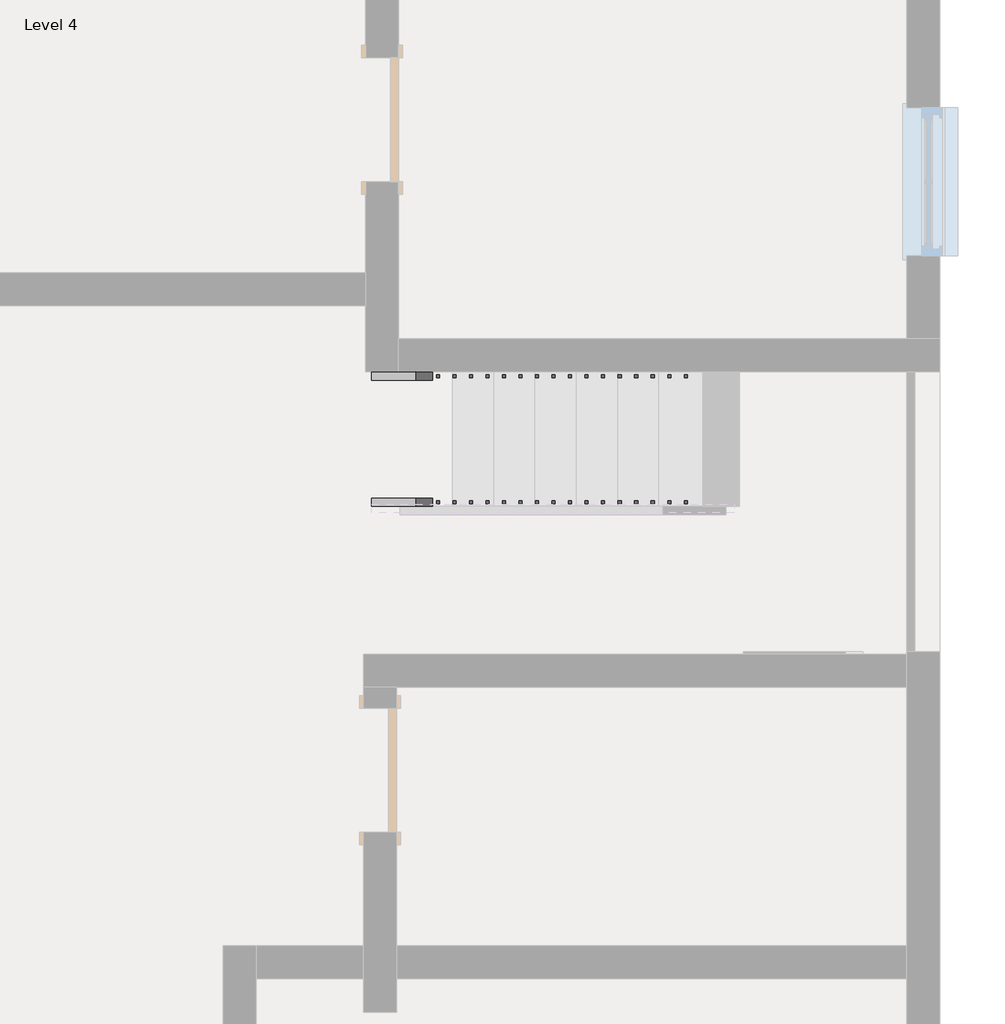
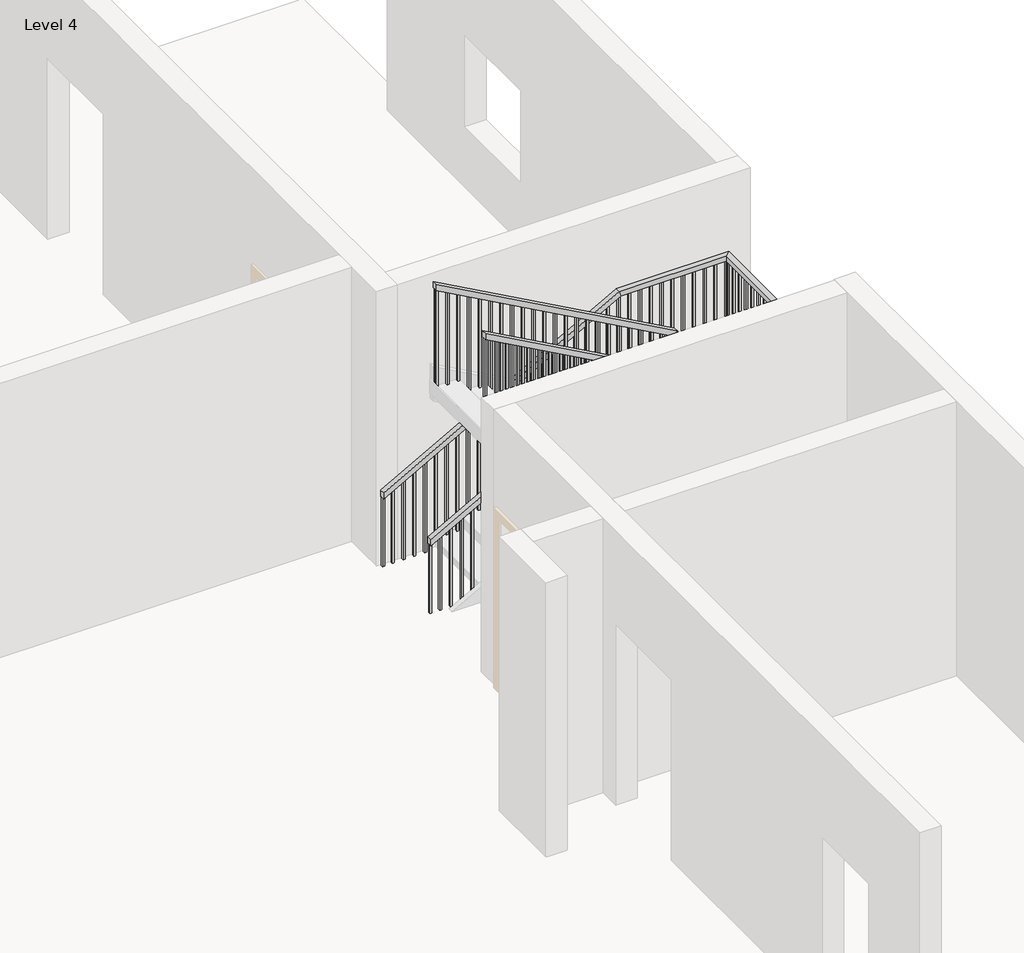
# One storey, part 3 of 4: 2 railings.
"""IFC4 building model written with IfcOpenShell, lengths in millimetres."""

from ifc_helpers import new_model, si_unit, frame, origin, place, context, project, spatial, polyline, outline, extrude, faceted_brep, element, save

model = new_model("IFC4")

# Units and contexts
model_context = context("Model", 3, world=origin())
ifc_project = project(units=[si_unit("LENGTHUNIT", "METRE", prefix="MILLI")], contexts=[model_context])

# Site, building, storey
site = spatial("IfcSite", under=ifc_project)
building = spatial("IfcBuilding", under=site)
storey = spatial("IfcBuildingStorey", under=building, Name="Level 4", Elevation=9144.0)

# Railings
placement = place(None, origin())
element("IfcRailing", 1, ObjectType="Handrail - Rectangular", at=placement, inside=storey, context=model_context, shape_type="SolidModel", body=[
    faceted_brep([(1537.1941283, 231.7547293, 10195.56), (1537.1941283, 231.7547293, 10137.4879132), (1537.1941283, 180.9547293, 10137.4879132), (1537.1941283, 180.9547293, 10195.56), (3765.8648053, 231.7547293, 11430.0), (3765.8648053, 180.9547293, 11430.0), (3765.8648053, 180.9547293, 11371.9279132), (3765.8648053, 231.7547293, 11371.9279132)], [[[0, 1, 2, 3]], [[4, 5, 6, 7]], [[1, 0, 4, 7]], [[2, 1, 7, 6]], [[3, 2, 6, 5]], [[0, 3, 5, 4]]]),
    faceted_brep([(3816.6648053, 231.7547293, 11430.0), (3816.6648053, 231.7547293, 11379.2), (3765.8648053, 231.7547293, 11379.2), (3765.8648053, 231.7547293, 11430.0), (3816.6648053, 142.8547293, 11430.0), (3765.8648053, 142.8547293, 11430.0), (3765.8648053, 92.0547293, 11379.2), (3816.6648053, 92.0547293, 11379.2)], [[[0, 1, 2, 3]], [[4, 5, 6, 7]], [[1, 0, 4, 7]], [[2, 1, 7, 6]], [[3, 2, 6, 5]], [[0, 3, 5, 4]]]),
    faceted_brep([(3816.6648053, 142.8547293, 11430.0), (3816.6648053, 92.0547293, 11379.2), (3765.8648053, 92.0547293, 11379.2), (3765.8648053, 142.8547293, 11430.0), (3816.6648053, 142.8547293, 11539.0223516), (3765.8648053, 142.8547293, 11509.0879132), (3765.8648053, 92.0547293, 11509.0879132), (3816.6648053, 92.0547293, 11539.0223516)], [[[0, 1, 2, 3]], [[4, 5, 6, 7]], [[1, 0, 4, 7]], [[2, 1, 7, 6]], [[3, 2, 6, 5]], [[0, 3, 5, 4]]]),
    faceted_brep([(3816.6648053, 92.0547293, 11539.0223516), (3765.8648053, 92.0547293, 11509.0879132), (3765.8648053, 142.8547293, 11509.0879132), (3816.6648053, 142.8547293, 11539.0223516), (1537.1941283, 92.0547293, 12801.6), (1537.1941283, 142.8547293, 12801.6), (1537.1941283, 142.8547293, 12743.5279132), (1537.1941283, 92.0547293, 12743.5279132)], [[[0, 1, 2, 3]], [[4, 5, 6, 7]], [[1, 0, 4, 7]], [[2, 1, 7, 6]], [[3, 2, 6, 5]], [[0, 3, 5, 4]]]),
    extrude(outline(polyline([(12727.7556667, 1565.5898053), (12738.3072849, 1546.5398053), (11750.04, 1546.5398053), (11750.04, 1565.5898053), (12727.7556667, 1565.5898053)])), frame((0.0, 107.9297293, 0.0), z_axis=(0.0, 1.0, 0.0), x_axis=(0.0, 0.0, 1.0)), (0.0, 0.0, 1.0), 19.05),
    extrude(outline(polyline([(12671.4803699, 1667.1898053), (12682.031988, 1648.1398053), (11750.04, 1648.1398053), (11750.04, 1667.1898053), (12671.4803699, 1667.1898053)])), frame((0.0, 107.9297293, 0.0), z_axis=(0.0, 1.0, 0.0), x_axis=(0.0, 0.0, 1.0)), (0.0, 0.0, 1.0), 19.05),
    extrude(outline(polyline([(12615.1609284, 1768.7898053), (12625.7125465, 1749.7398053), (11750.04, 1749.7398053), (11750.04, 1768.7898053), (12615.1609284, 1768.7898053)])), frame((0.0, 107.9297293, 0.0), z_axis=(0.0, 1.0, 0.0), x_axis=(0.0, 0.0, 1.0)), (0.0, 0.0, 1.0), 19.05),
    extrude(outline(polyline([(12558.9297761, 1870.3898053), (12569.4813943, 1851.3398053), (11612.88, 1851.3398053), (11612.88, 1870.3898053), (12558.9297761, 1870.3898053)])), frame((0.0, 107.9297293, 0.0), z_axis=(0.0, 1.0, 0.0), x_axis=(0.0, 0.0, 1.0)), (0.0, 0.0, 1.0), 19.05),
    extrude(outline(polyline([(12502.6544792, 1971.9898053), (12513.2060974, 1952.9398053), (11612.88, 1952.9398053), (11612.88, 1971.9898053), (12502.6544792, 1971.9898053)])), frame((0.0, 107.9297293, 0.0), z_axis=(0.0, 1.0, 0.0), x_axis=(0.0, 0.0, 1.0)), (0.0, 0.0, 1.0), 19.05),
    extrude(outline(polyline([(12446.3791823, 2073.5898053), (12456.9308005, 2054.5398053), (11475.72, 2054.5398053), (11475.72, 2073.5898053), (12446.3791823, 2073.5898053)])), frame((0.0, 107.9297293, 0.0), z_axis=(0.0, 1.0, 0.0), x_axis=(0.0, 0.0, 1.0)), (0.0, 0.0, 1.0), 19.05),
    extrude(outline(polyline([(12390.1038855, 2175.1898053), (12400.6555036, 2156.1398053), (11475.72, 2156.1398053), (11475.72, 2175.1898053), (12390.1038855, 2175.1898053)])), frame((0.0, 107.9297293, 0.0), z_axis=(0.0, 1.0, 0.0), x_axis=(0.0, 0.0, 1.0)), (0.0, 0.0, 1.0), 19.05),
    extrude(outline(polyline([(12333.8285886, 2276.7898053), (12344.3802067, 2257.7398053), (11475.72, 2257.7398053), (11475.72, 2276.7898053), (12333.8285886, 2276.7898053)])), frame((0.0, 107.9297293, 0.0), z_axis=(0.0, 1.0, 0.0), x_axis=(0.0, 0.0, 1.0)), (0.0, 0.0, 1.0), 19.05),
    extrude(outline(polyline([(12277.5532917, 2378.3898053), (12288.1049099, 2359.3398053), (11338.56, 2359.3398053), (11338.56, 2378.3898053), (12277.5532917, 2378.3898053)])), frame((0.0, 107.9297293, 0.0), z_axis=(0.0, 1.0, 0.0), x_axis=(0.0, 0.0, 1.0)), (0.0, 0.0, 1.0), 19.05),
    extrude(outline(polyline([(12221.2779948, 2479.9898053), (12231.829613, 2460.9398053), (11338.56, 2460.9398053), (11338.56, 2479.9898053), (12221.2779948, 2479.9898053)])), frame((0.0, 107.9297293, 0.0), z_axis=(0.0, 1.0, 0.0), x_axis=(0.0, 0.0, 1.0)), (0.0, 0.0, 1.0), 19.05),
    extrude(outline(polyline([(12165.0026979, 2581.5898053), (12175.5543161, 2562.5398053), (11201.4, 2562.5398053), (11201.4, 2581.5898053), (12165.0026979, 2581.5898053)])), frame((0.0, 107.9297293, 0.0), z_axis=(0.0, 1.0, 0.0), x_axis=(0.0, 0.0, 1.0)), (0.0, 0.0, 1.0), 19.05),
    extrude(outline(polyline([(12108.727401, 2683.1898053), (12119.2790192, 2664.1398053), (11201.4, 2664.1398053), (11201.4, 2683.1898053), (12108.727401, 2683.1898053)])), frame((0.0, 107.9297293, 0.0), z_axis=(0.0, 1.0, 0.0), x_axis=(0.0, 0.0, 1.0)), (0.0, 0.0, 1.0), 19.05),
    extrude(outline(polyline([(12052.4962488, 2784.7898053), (12063.0478669, 2765.7398053), (11201.4, 2765.7398053), (11201.4, 2784.7898053), (12052.4962488, 2784.7898053)])), frame((0.0, 107.9297293, 0.0), z_axis=(0.0, 1.0, 0.0), x_axis=(0.0, 0.0, 1.0)), (0.0, 0.0, 1.0), 19.05),
    extrude(outline(polyline([(11996.2209519, 2886.3898053), (12006.77257, 2867.3398053), (11064.24, 2867.3398053), (11064.24, 2886.3898053), (11996.2209519, 2886.3898053)])), frame((0.0, 107.9297293, 0.0), z_axis=(0.0, 1.0, 0.0), x_axis=(0.0, 0.0, 1.0)), (0.0, 0.0, 1.0), 19.05),
    extrude(outline(polyline([(11939.945655, 2987.9898053), (11950.4972732, 2968.9398053), (11064.24, 2968.9398053), (11064.24, 2987.9898053), (11939.945655, 2987.9898053)])), frame((0.0, 107.9297293, 0.0), z_axis=(0.0, 1.0, 0.0), x_axis=(0.0, 0.0, 1.0)), (0.0, 0.0, 1.0), 19.05),
    extrude(outline(polyline([(11883.6703581, 3089.5898053), (11894.2219763, 3070.5398053), (10927.08, 3070.5398053), (10927.08, 3089.5898053), (11883.6703581, 3089.5898053)])), frame((0.0, 107.9297293, 0.0), z_axis=(0.0, 1.0, 0.0), x_axis=(0.0, 0.0, 1.0)), (0.0, 0.0, 1.0), 19.05),
    extrude(outline(polyline([(11827.3950612, 3191.1898053), (11837.9466794, 3172.1398053), (10927.08, 3172.1398053), (10927.08, 3191.1898053), (11827.3950612, 3191.1898053)])), frame((0.0, 107.9297293, 0.0), z_axis=(0.0, 1.0, 0.0), x_axis=(0.0, 0.0, 1.0)), (0.0, 0.0, 1.0), 19.05),
    extrude(outline(polyline([(11771.1197643, 3292.7898053), (11781.6713825, 3273.7398053), (10927.08, 3273.7398053), (10927.08, 3292.7898053), (11771.1197643, 3292.7898053)])), frame((0.0, 107.9297293, 0.0), z_axis=(0.0, 1.0, 0.0), x_axis=(0.0, 0.0, 1.0)), (0.0, 0.0, 1.0), 19.05),
    extrude(outline(polyline([(11714.8444675, 3394.3898053), (11725.3960856, 3375.3398053), (10789.92, 3375.3398053), (10789.92, 3394.3898053), (11714.8444675, 3394.3898053)])), frame((0.0, 107.9297293, 0.0), z_axis=(0.0, 1.0, 0.0), x_axis=(0.0, 0.0, 1.0)), (0.0, 0.0, 1.0), 19.05),
    extrude(outline(polyline([(11658.5691706, 3495.9898053), (11669.1207888, 3476.9398053), (10789.92, 3476.9398053), (10789.92, 3495.9898053), (11658.5691706, 3495.9898053)])), frame((0.0, 107.9297293, 0.0), z_axis=(0.0, 1.0, 0.0), x_axis=(0.0, 0.0, 1.0)), (0.0, 0.0, 1.0), 19.05),
    extrude(outline(polyline([(11602.2938737, 3597.5898053), (11612.8454919, 3578.5398053), (10652.76, 3578.5398053), (10652.76, 3597.5898053), (11602.2938737, 3597.5898053)])), frame((0.0, 107.9297293, 0.0), z_axis=(0.0, 1.0, 0.0), x_axis=(0.0, 0.0, 1.0)), (0.0, 0.0, 1.0), 19.05),
    extrude(outline(polyline([(11546.0185768, 3699.1898053), (11556.570195, 3680.1398053), (10652.76, 3680.1398053), (10652.76, 3699.1898053), (11546.0185768, 3699.1898053)])), frame((0.0, 107.9297293, 0.0), z_axis=(0.0, 1.0, 0.0), x_axis=(0.0, 0.0, 1.0)), (0.0, 0.0, 1.0), 19.05),
    extrude(outline(polyline([(11380.8202537, 3781.9191283), (11370.2686355, 3762.8691283), (10515.6, 3762.8691283), (10515.6, 3781.9191283), (11380.8202537, 3781.9191283)])), frame((0.0, 196.8297293, 0.0), z_axis=(0.0, 1.0, 0.0), x_axis=(0.0, 0.0, 1.0)), (0.0, 0.0, 1.0), 19.05),
    extrude(outline(polyline([(11324.5449568, 3680.3191283), (11313.9933387, 3661.2691283), (10378.44, 3661.2691283), (10378.44, 3680.3191283), (11324.5449568, 3680.3191283)])), frame((0.0, 196.8297293, 0.0), z_axis=(0.0, 1.0, 0.0), x_axis=(0.0, 0.0, 1.0)), (0.0, 0.0, 1.0), 19.05),
    extrude(outline(polyline([(11268.2696599, 3578.7191283), (11257.7180418, 3559.6691283), (10378.44, 3559.6691283), (10378.44, 3578.7191283), (11268.2696599, 3578.7191283)])), frame((0.0, 196.8297293, 0.0), z_axis=(0.0, 1.0, 0.0), x_axis=(0.0, 0.0, 1.0)), (0.0, 0.0, 1.0), 19.05),
    extrude(outline(polyline([(11211.9943631, 3477.1191283), (11201.4427449, 3458.0691283), (10241.28, 3458.0691283), (10241.28, 3477.1191283), (11211.9943631, 3477.1191283)])), frame((0.0, 196.8297293, 0.0), z_axis=(0.0, 1.0, 0.0), x_axis=(0.0, 0.0, 1.0)), (0.0, 0.0, 1.0), 19.05),
    extrude(outline(polyline([(11155.7190662, 3375.5191283), (11145.167448, 3356.4691283), (10241.28, 3356.4691283), (10241.28, 3375.5191283), (11155.7190662, 3375.5191283)])), frame((0.0, 196.8297293, 0.0), z_axis=(0.0, 1.0, 0.0), x_axis=(0.0, 0.0, 1.0)), (0.0, 0.0, 1.0), 19.05),
    extrude(outline(polyline([(11099.4437693, 3273.9191283), (11088.8921511, 3254.8691283), (10104.12, 3254.8691283), (10104.12, 3273.9191283), (11099.4437693, 3273.9191283)])), frame((0.0, 196.8297293, 0.0), z_axis=(0.0, 1.0, 0.0), x_axis=(0.0, 0.0, 1.0)), (0.0, 0.0, 1.0), 19.05),
    extrude(outline(polyline([(11043.1684724, 3172.3191283), (11032.6168543, 3153.2691283), (10104.12, 3153.2691283), (10104.12, 3172.3191283), (11043.1684724, 3172.3191283)])), frame((0.0, 196.8297293, 0.0), z_axis=(0.0, 1.0, 0.0), x_axis=(0.0, 0.0, 1.0)), (0.0, 0.0, 1.0), 19.05),
    extrude(outline(polyline([(10986.8931755, 3070.7191283), (10976.3415574, 3051.6691283), (10104.12, 3051.6691283), (10104.12, 3070.7191283), (10986.8931755, 3070.7191283)])), frame((0.0, 196.8297293, 0.0), z_axis=(0.0, 1.0, 0.0), x_axis=(0.0, 0.0, 1.0)), (0.0, 0.0, 1.0), 19.05),
    extrude(outline(polyline([(10930.6178787, 2969.1191283), (10920.0662605, 2950.0691283), (9966.96, 2950.0691283), (9966.96, 2969.1191283), (10930.6178787, 2969.1191283)])), frame((0.0, 196.8297293, 0.0), z_axis=(0.0, 1.0, 0.0), x_axis=(0.0, 0.0, 1.0)), (0.0, 0.0, 1.0), 19.05),
    extrude(outline(polyline([(10874.3425818, 2867.5191283), (10863.7909636, 2848.4691283), (9966.96, 2848.4691283), (9966.96, 2867.5191283), (10874.3425818, 2867.5191283)])), frame((0.0, 196.8297293, 0.0), z_axis=(0.0, 1.0, 0.0), x_axis=(0.0, 0.0, 1.0)), (0.0, 0.0, 1.0), 19.05),
    extrude(outline(polyline([(10818.0672849, 2765.9191283), (10807.5156667, 2746.8691283), (9829.8, 2746.8691283), (9829.8, 2765.9191283), (10818.0672849, 2765.9191283)])), frame((0.0, 196.8297293, 0.0), z_axis=(0.0, 1.0, 0.0), x_axis=(0.0, 0.0, 1.0)), (0.0, 0.0, 1.0), 19.05),
    extrude(outline(polyline([(10761.791988, 2664.3191283), (10751.2403699, 2645.2691283), (9829.8, 2645.2691283), (9829.8, 2664.3191283), (10761.791988, 2664.3191283)])), frame((0.0, 196.8297293, 0.0), z_axis=(0.0, 1.0, 0.0), x_axis=(0.0, 0.0, 1.0)), (0.0, 0.0, 1.0), 19.05),
    extrude(outline(polyline([(10705.4725466, 2562.7191283), (10694.9209284, 2543.6691283), (9829.8, 2543.6691283), (9829.8, 2562.7191283), (10705.4725466, 2562.7191283)])), frame((0.0, 196.8297293, 0.0), z_axis=(0.0, 1.0, 0.0), x_axis=(0.0, 0.0, 1.0)), (0.0, 0.0, 1.0), 19.05),
    extrude(outline(polyline([(10649.2413943, 2461.1191283), (10638.6897761, 2442.0691283), (9692.64, 2442.0691283), (9692.64, 2461.1191283), (10649.2413943, 2461.1191283)])), frame((0.0, 196.8297293, 0.0), z_axis=(0.0, 1.0, 0.0), x_axis=(0.0, 0.0, 1.0)), (0.0, 0.0, 1.0), 19.05),
    extrude(outline(polyline([(10592.9660974, 2359.5191283), (10582.4144792, 2340.4691283), (9692.64, 2340.4691283), (9692.64, 2359.5191283), (10592.9660974, 2359.5191283)])), frame((0.0, 196.8297293, 0.0), z_axis=(0.0, 1.0, 0.0), x_axis=(0.0, 0.0, 1.0)), (0.0, 0.0, 1.0), 19.05),
    extrude(outline(polyline([(10536.6908005, 2257.9191283), (10526.1391823, 2238.8691283), (9555.48, 2238.8691283), (9555.48, 2257.9191283), (10536.6908005, 2257.9191283)])), frame((0.0, 196.8297293, 0.0), z_axis=(0.0, 1.0, 0.0), x_axis=(0.0, 0.0, 1.0)), (0.0, 0.0, 1.0), 19.05),
    extrude(outline(polyline([(10480.4155036, 2156.3191283), (10469.8638855, 2137.2691283), (9555.48, 2137.2691283), (9555.48, 2156.3191283), (10480.4155036, 2156.3191283)])), frame((0.0, 196.8297293, 0.0), z_axis=(0.0, 1.0, 0.0), x_axis=(0.0, 0.0, 1.0)), (0.0, 0.0, 1.0), 19.05),
    extrude(outline(polyline([(10424.1402067, 2054.7191283), (10413.5885886, 2035.6691283), (9555.48, 2035.6691283), (9555.48, 2054.7191283), (10424.1402067, 2054.7191283)])), frame((0.0, 196.8297293, 0.0), z_axis=(0.0, 1.0, 0.0), x_axis=(0.0, 0.0, 1.0)), (0.0, 0.0, 1.0), 19.05),
    extrude(outline(polyline([(10367.8649099, 1953.1191283), (10357.3132917, 1934.0691283), (9418.32, 1934.0691283), (9418.32, 1953.1191283), (10367.8649099, 1953.1191283)])), frame((0.0, 196.8297293, 0.0), z_axis=(0.0, 1.0, 0.0), x_axis=(0.0, 0.0, 1.0)), (0.0, 0.0, 1.0), 19.05),
    extrude(outline(polyline([(10311.589613, 1851.5191283), (10301.0379948, 1832.4691283), (9418.32, 1832.4691283), (9418.32, 1851.5191283), (10311.589613, 1851.5191283)])), frame((0.0, 196.8297293, 0.0), z_axis=(0.0, 1.0, 0.0), x_axis=(0.0, 0.0, 1.0)), (0.0, 0.0, 1.0), 19.05),
    extrude(outline(polyline([(10255.3143161, 1749.9191283), (10244.7626979, 1730.8691283), (9281.16, 1730.8691283), (9281.16, 1749.9191283), (10255.3143161, 1749.9191283)])), frame((0.0, 196.8297293, 0.0), z_axis=(0.0, 1.0, 0.0), x_axis=(0.0, 0.0, 1.0)), (0.0, 0.0, 1.0), 19.05),
    extrude(outline(polyline([(10199.0390192, 1648.3191283), (10188.487401, 1629.2691283), (9281.16, 1629.2691283), (9281.16, 1648.3191283), (10199.0390192, 1648.3191283)])), frame((0.0, 196.8297293, 0.0), z_axis=(0.0, 1.0, 0.0), x_axis=(0.0, 0.0, 1.0)), (0.0, 0.0, 1.0), 19.05),
    extrude(outline(polyline([(3781.7398053, 126.9797293), (3800.7898053, 126.9797293), (3800.7898053, 107.9297293), (3781.7398053, 107.9297293), (3781.7398053, 126.9797293)])), frame((0.0, 0.0, 10515.6), z_axis=(0.0, 0.0, 1.0), x_axis=(1.0, 0.0, 0.0)), (0.0, 0.0, 1.0), 863.6),
    extrude(outline(polyline([(11391.2725465, 3800.7898053), (11380.7209284, 3781.7398053), (10515.6, 3781.7398053), (10515.6, 3800.7898053), (11391.2725465, 3800.7898053)])), frame((0.0, 196.8297293, 0.0), z_axis=(0.0, 1.0, 0.0), x_axis=(0.0, 0.0, 1.0)), (0.0, 0.0, 1.0), 19.05),
    extrude(outline(polyline([(12732.9762951, 1556.2441283), (12743.5279132, 1537.1941283), (11750.04, 1537.1941283), (11750.04, 1556.2441283), (12732.9762951, 1556.2441283)])), frame((0.0, 107.9297293, 0.0), z_axis=(0.0, 1.0, 0.0), x_axis=(0.0, 0.0, 1.0)), (0.0, 0.0, 1.0), 19.05),
    extrude(outline(polyline([(10148.0395314, 1556.2441283), (10137.4879132, 1537.1941283), (9281.16, 1537.1941283), (9281.16, 1556.2441283), (10148.0395314, 1556.2441283)])), frame((0.0, 196.8297293, 0.0), z_axis=(0.0, 1.0, 0.0), x_axis=(0.0, 0.0, 1.0)), (0.0, 0.0, 1.0), 19.05),
])
element("IfcRailing", 2, ObjectType="Handrail - Rectangular", at=placement, inside=storey, context=model_context, shape_type="SolidModel", body=[
    faceted_brep([(1537.1941283, 1006.4547293, 10195.56), (1537.1941283, 1006.4547293, 10137.4879132), (1537.1941283, 955.6547293, 10137.4879132), (1537.1941283, 955.6547293, 10195.56), (3765.8648053, 1006.4547293, 11430.0), (3778.9939056, 1006.4547293, 11379.2), (3778.9939056, 955.6547293, 11379.2), (3765.8648053, 955.6547293, 11430.0), (4826.4941283, 1006.4547293, 11430.0), (4826.4941283, 1006.4547293, 11379.2), (4775.6941283, 955.6547293, 11379.2), (4775.6941283, 955.6547293, 11430.0), (4826.4941283, -714.2964201, 11430.0), (4826.4941283, -714.2964201, 11379.2), (4775.6941283, -663.4964201, 11379.2), (4775.6941283, -663.4964201, 11430.0), (4013.4948805, -714.2964201, 11430.0), (4000.3657803, -714.2964201, 11379.2), (4000.3657803, -663.4964201, 11379.2), (4013.4948805, -663.4964201, 11430.0), (1537.1941283, -714.2964201, 12801.6), (1537.1941283, -663.4964201, 12801.6), (1537.1941283, -663.4964201, 12743.5279132), (1537.1941283, -714.2964201, 12743.5279132)], [[[0, 1, 2, 3]], [[1, 0, 4, 5]], [[2, 1, 5, 6]], [[3, 2, 6, 7]], [[0, 3, 7, 4]], [[5, 4, 8, 9]], [[6, 5, 9, 10]], [[7, 6, 10, 11]], [[4, 7, 11, 8]], [[9, 8, 12, 13]], [[10, 9, 13, 14]], [[11, 10, 14, 15]], [[8, 11, 15, 12]], [[13, 12, 16, 17]], [[14, 13, 17, 18]], [[15, 14, 18, 19]], [[12, 15, 19, 16]], [[20, 21, 22, 23]], [[17, 16, 20, 23]], [[18, 17, 23, 22]], [[19, 18, 22, 21]], [[16, 19, 21, 20]]]),
    extrude(outline(polyline([(12741.7693102, 1540.3691283), (11750.04, 1540.3691283), (11750.04, 1559.4191283), (12731.2176921, 1559.4191283), (12741.7693102, 1540.3691283)])), frame((0.0, -698.4214201, 0.0), z_axis=(0.0, 1.0, 0.0), x_axis=(0.0, 0.0, 1.0)), (0.0, 0.0, 1.0), 19.05),
    extrude(outline(polyline([(12685.4940133, 1641.9691283), (11750.04, 1641.9691283), (11750.04, 1661.0191283), (12674.9423952, 1661.0191283), (12685.4940133, 1641.9691283)])), frame((0.0, -698.4214201, 0.0), z_axis=(0.0, 1.0, 0.0), x_axis=(0.0, 0.0, 1.0)), (0.0, 0.0, 1.0), 19.05),
    extrude(outline(polyline([(12629.2187165, 1743.5691283), (11750.04, 1743.5691283), (11750.04, 1762.6191283), (12618.6670983, 1762.6191283), (12629.2187165, 1743.5691283)])), frame((0.0, -698.4214201, 0.0), z_axis=(0.0, 1.0, 0.0), x_axis=(0.0, 0.0, 1.0)), (0.0, 0.0, 1.0), 19.05),
    extrude(outline(polyline([(12572.9434196, 1845.1691283), (11612.88, 1845.1691283), (11612.88, 1864.2191283), (12562.3918014, 1864.2191283), (12572.9434196, 1845.1691283)])), frame((0.0, -698.4214201, 0.0), z_axis=(0.0, 1.0, 0.0), x_axis=(0.0, 0.0, 1.0)), (0.0, 0.0, 1.0), 19.05),
    extrude(outline(polyline([(12516.6681227, 1946.7691283), (11612.88, 1946.7691283), (11612.88, 1965.8191283), (12506.1165045, 1965.8191283), (12516.6681227, 1946.7691283)])), frame((0.0, -698.4214201, 0.0), z_axis=(0.0, 1.0, 0.0), x_axis=(0.0, 0.0, 1.0)), (0.0, 0.0, 1.0), 19.05),
    extrude(outline(polyline([(12460.3928258, 2048.3691283), (11475.72, 2048.3691283), (11475.72, 2067.4191283), (12449.8412076, 2067.4191283), (12460.3928258, 2048.3691283)])), frame((0.0, -698.4214201, 0.0), z_axis=(0.0, 1.0, 0.0), x_axis=(0.0, 0.0, 1.0)), (0.0, 0.0, 1.0), 19.05),
    extrude(outline(polyline([(12404.1175289, 2149.9691283), (11475.72, 2149.9691283), (11475.72, 2169.0191283), (12393.5659108, 2169.0191283), (12404.1175289, 2149.9691283)])), frame((0.0, -698.4214201, 0.0), z_axis=(0.0, 1.0, 0.0), x_axis=(0.0, 0.0, 1.0)), (0.0, 0.0, 1.0), 19.05),
    extrude(outline(polyline([(12347.8422321, 2251.5691283), (11475.72, 2251.5691283), (11475.72, 2270.6191283), (12337.2906139, 2270.6191283), (12347.8422321, 2251.5691283)])), frame((0.0, -698.4214201, 0.0), z_axis=(0.0, 1.0, 0.0), x_axis=(0.0, 0.0, 1.0)), (0.0, 0.0, 1.0), 19.05),
    extrude(outline(polyline([(12291.5669352, 2353.1691283), (11338.56, 2353.1691283), (11338.56, 2372.2191283), (12281.015317, 2372.2191283), (12291.5669352, 2353.1691283)])), frame((0.0, -698.4214201, 0.0), z_axis=(0.0, 1.0, 0.0), x_axis=(0.0, 0.0, 1.0)), (0.0, 0.0, 1.0), 19.05),
    extrude(outline(polyline([(12235.2916383, 2454.7691283), (11338.56, 2454.7691283), (11338.56, 2473.8191283), (12224.7400201, 2473.8191283), (12235.2916383, 2454.7691283)])), frame((0.0, -698.4214201, 0.0), z_axis=(0.0, 1.0, 0.0), x_axis=(0.0, 0.0, 1.0)), (0.0, 0.0, 1.0), 19.05),
    extrude(outline(polyline([(12179.0163414, 2556.3691283), (11201.4, 2556.3691283), (11201.4, 2575.4191283), (12168.4647232, 2575.4191283), (12179.0163414, 2556.3691283)])), frame((0.0, -698.4214201, 0.0), z_axis=(0.0, 1.0, 0.0), x_axis=(0.0, 0.0, 1.0)), (0.0, 0.0, 1.0), 19.05),
    extrude(outline(polyline([(12122.7410445, 2657.9691283), (11201.4, 2657.9691283), (11201.4, 2677.0191283), (12112.1894264, 2677.0191283), (12122.7410445, 2657.9691283)])), frame((0.0, -698.4214201, 0.0), z_axis=(0.0, 1.0, 0.0), x_axis=(0.0, 0.0, 1.0)), (0.0, 0.0, 1.0), 19.05),
    extrude(outline(polyline([(12066.4657476, 2759.5691283), (11201.4, 2759.5691283), (11201.4, 2778.6191283), (12055.9141295, 2778.6191283), (12066.4657476, 2759.5691283)])), frame((0.0, -698.4214201, 0.0), z_axis=(0.0, 1.0, 0.0), x_axis=(0.0, 0.0, 1.0)), (0.0, 0.0, 1.0), 19.05),
    extrude(outline(polyline([(12010.3449568, 2861.1691283), (11064.24, 2861.1691283), (11064.24, 2880.2191283), (11999.7933387, 2880.2191283), (12010.3449568, 2861.1691283)])), frame((0.0, -698.4214201, 0.0), z_axis=(0.0, 1.0, 0.0), x_axis=(0.0, 0.0, 1.0)), (0.0, 0.0, 1.0), 19.05),
    extrude(outline(polyline([(11954.0696599, 2962.7691283), (11064.24, 2962.7691283), (11064.24, 2981.8191283), (11943.5180418, 2981.8191283), (11954.0696599, 2962.7691283)])), frame((0.0, -698.4214201, 0.0), z_axis=(0.0, 1.0, 0.0), x_axis=(0.0, 0.0, 1.0)), (0.0, 0.0, 1.0), 19.05),
    extrude(outline(polyline([(11897.7943631, 3064.3691283), (10927.08, 3064.3691283), (10927.08, 3083.4191283), (11887.2427449, 3083.4191283), (11897.7943631, 3064.3691283)])), frame((0.0, -698.4214201, 0.0), z_axis=(0.0, 1.0, 0.0), x_axis=(0.0, 0.0, 1.0)), (0.0, 0.0, 1.0), 19.05),
    extrude(outline(polyline([(11841.5190662, 3165.9691283), (10927.08, 3165.9691283), (10927.08, 3185.0191283), (11830.967448, 3185.0191283), (11841.5190662, 3165.9691283)])), frame((0.0, -698.4214201, 0.0), z_axis=(0.0, 1.0, 0.0), x_axis=(0.0, 0.0, 1.0)), (0.0, 0.0, 1.0), 19.05),
    extrude(outline(polyline([(11785.0892632, 3267.5691283), (10927.08, 3267.5691283), (10927.08, 3286.6191283), (11774.5376451, 3286.6191283), (11785.0892632, 3267.5691283)])), frame((0.0, -698.4214201, 0.0), z_axis=(0.0, 1.0, 0.0), x_axis=(0.0, 0.0, 1.0)), (0.0, 0.0, 1.0), 19.05),
    extrude(outline(polyline([(11728.9684724, 3369.1691283), (10789.92, 3369.1691283), (10789.92, 3388.2191283), (11718.4168543, 3388.2191283), (11728.9684724, 3369.1691283)])), frame((0.0, -698.4214201, 0.0), z_axis=(0.0, 1.0, 0.0), x_axis=(0.0, 0.0, 1.0)), (0.0, 0.0, 1.0), 19.05),
    extrude(outline(polyline([(11672.6931755, 3470.7691283), (10789.92, 3470.7691283), (10789.92, 3489.8191283), (11662.1415574, 3489.8191283), (11672.6931755, 3470.7691283)])), frame((0.0, -698.4214201, 0.0), z_axis=(0.0, 1.0, 0.0), x_axis=(0.0, 0.0, 1.0)), (0.0, 0.0, 1.0), 19.05),
    extrude(outline(polyline([(11616.4178787, 3572.3691283), (10652.76, 3572.3691283), (10652.76, 3591.4191283), (11605.8662605, 3591.4191283), (11616.4178787, 3572.3691283)])), frame((0.0, -698.4214201, 0.0), z_axis=(0.0, 1.0, 0.0), x_axis=(0.0, 0.0, 1.0)), (0.0, 0.0, 1.0), 19.05),
    extrude(outline(polyline([(11560.1425818, 3673.9691283), (10652.76, 3673.9691283), (10652.76, 3693.0191283), (11549.5909636, 3693.0191283), (11560.1425818, 3673.9691283)])), frame((0.0, -698.4214201, 0.0), z_axis=(0.0, 1.0, 0.0), x_axis=(0.0, 0.0, 1.0)), (0.0, 0.0, 1.0), 19.05),
    extrude(outline(polyline([(11503.8672849, 3775.5691283), (10515.6, 3775.5691283), (10515.6, 3794.6191283), (11493.3156667, 3794.6191283), (11503.8672849, 3775.5691283)])), frame((0.0, -698.4214201, 0.0), z_axis=(0.0, 1.0, 0.0), x_axis=(0.0, 0.0, 1.0)), (0.0, 0.0, 1.0), 19.05),
    extrude(outline(polyline([(11447.591988, 3877.1691283), (10515.6, 3877.1691283), (10515.6, 3896.2191283), (11437.0403699, 3896.2191283), (11447.591988, 3877.1691283)])), frame((0.0, -698.4214201, 0.0), z_axis=(0.0, 1.0, 0.0), x_axis=(0.0, 0.0, 1.0)), (0.0, 0.0, 1.0), 19.05),
    extrude(outline(polyline([(11391.3166911, 3978.7691283), (10515.6, 3978.7691283), (10515.6, 3997.8191283), (11380.765073, 3997.8191283), (11391.3166911, 3978.7691283)])), frame((0.0, -698.4214201, 0.0), z_axis=(0.0, 1.0, 0.0), x_axis=(0.0, 0.0, 1.0)), (0.0, 0.0, 1.0), 19.05),
    extrude(outline(polyline([(4099.4191283, -698.4214201), (4080.3691283, -698.4214201), (4080.3691283, -679.3714201), (4099.4191283, -679.3714201), (4099.4191283, -698.4214201)])), frame((0.0, 0.0, 10515.6), z_axis=(0.0, 0.0, 1.0), x_axis=(1.0, 0.0, 0.0)), (0.0, 0.0, 1.0), 863.6),
    extrude(outline(polyline([(4201.0191283, -698.4214201), (4181.9691283, -698.4214201), (4181.9691283, -679.3714201), (4201.0191283, -679.3714201), (4201.0191283, -698.4214201)])), frame((0.0, 0.0, 10515.6), z_axis=(0.0, 0.0, 1.0), x_axis=(1.0, 0.0, 0.0)), (0.0, 0.0, 1.0), 863.6),
    extrude(outline(polyline([(4302.6191283, -698.4214201), (4283.5691283, -698.4214201), (4283.5691283, -679.3714201), (4302.6191283, -679.3714201), (4302.6191283, -698.4214201)])), frame((0.0, 0.0, 10515.6), z_axis=(0.0, 0.0, 1.0), x_axis=(1.0, 0.0, 0.0)), (0.0, 0.0, 1.0), 863.6),
    extrude(outline(polyline([(4404.2191283, -698.4214201), (4385.1691283, -698.4214201), (4385.1691283, -679.3714201), (4404.2191283, -679.3714201), (4404.2191283, -698.4214201)])), frame((0.0, 0.0, 10515.6), z_axis=(0.0, 0.0, 1.0), x_axis=(1.0, 0.0, 0.0)), (0.0, 0.0, 1.0), 863.6),
    extrude(outline(polyline([(4505.8191283, -698.4214201), (4486.7691283, -698.4214201), (4486.7691283, -679.3714201), (4505.8191283, -679.3714201), (4505.8191283, -698.4214201)])), frame((0.0, 0.0, 10515.6), z_axis=(0.0, 0.0, 1.0), x_axis=(1.0, 0.0, 0.0)), (0.0, 0.0, 1.0), 863.6),
    extrude(outline(polyline([(4607.4191283, -698.4214201), (4588.3691283, -698.4214201), (4588.3691283, -679.3714201), (4607.4191283, -679.3714201), (4607.4191283, -698.4214201)])), frame((0.0, 0.0, 10515.6), z_axis=(0.0, 0.0, 1.0), x_axis=(1.0, 0.0, 0.0)), (0.0, 0.0, 1.0), 863.6),
    extrude(outline(polyline([(4709.0191283, -698.4214201), (4689.9691283, -698.4214201), (4689.9691283, -679.3714201), (4709.0191283, -679.3714201), (4709.0191283, -698.4214201)])), frame((0.0, 0.0, 10515.6), z_axis=(0.0, 0.0, 1.0), x_axis=(1.0, 0.0, 0.0)), (0.0, 0.0, 1.0), 863.6),
    extrude(outline(polyline([(4810.6191283, -635.0202707), (4810.6191283, -654.0702707), (4791.5691283, -654.0702707), (4791.5691283, -635.0202707), (4810.6191283, -635.0202707)])), frame((0.0, 0.0, 10515.6), z_axis=(0.0, 0.0, 1.0), x_axis=(1.0, 0.0, 0.0)), (0.0, 0.0, 1.0), 863.6),
    extrude(outline(polyline([(4810.6191283, -533.4202707), (4810.6191283, -552.4702707), (4791.5691283, -552.4702707), (4791.5691283, -533.4202707), (4810.6191283, -533.4202707)])), frame((0.0, 0.0, 10515.6), z_axis=(0.0, 0.0, 1.0), x_axis=(1.0, 0.0, 0.0)), (0.0, 0.0, 1.0), 863.6),
    extrude(outline(polyline([(4810.6191283, -431.8202707), (4810.6191283, -450.8702707), (4791.5691283, -450.8702707), (4791.5691283, -431.8202707), (4810.6191283, -431.8202707)])), frame((0.0, 0.0, 10515.6), z_axis=(0.0, 0.0, 1.0), x_axis=(1.0, 0.0, 0.0)), (0.0, 0.0, 1.0), 863.6),
    extrude(outline(polyline([(4810.6191283, -330.2202707), (4810.6191283, -349.2702707), (4791.5691283, -349.2702707), (4791.5691283, -330.2202707), (4810.6191283, -330.2202707)])), frame((0.0, 0.0, 10515.6), z_axis=(0.0, 0.0, 1.0), x_axis=(1.0, 0.0, 0.0)), (0.0, 0.0, 1.0), 863.6),
    extrude(outline(polyline([(4810.6191283, -228.6202707), (4810.6191283, -247.6702707), (4791.5691283, -247.6702707), (4791.5691283, -228.6202707), (4810.6191283, -228.6202707)])), frame((0.0, 0.0, 10515.6), z_axis=(0.0, 0.0, 1.0), x_axis=(1.0, 0.0, 0.0)), (0.0, 0.0, 1.0), 863.6),
    extrude(outline(polyline([(4810.6191283, -127.0202707), (4810.6191283, -146.0702707), (4791.5691283, -146.0702707), (4791.5691283, -127.0202707), (4810.6191283, -127.0202707)])), frame((0.0, 0.0, 10515.6), z_axis=(0.0, 0.0, 1.0), x_axis=(1.0, 0.0, 0.0)), (0.0, 0.0, 1.0), 863.6),
    extrude(outline(polyline([(4810.6191283, -25.4202707), (4810.6191283, -44.4702707), (4791.5691283, -44.4702707), (4791.5691283, -25.4202707), (4810.6191283, -25.4202707)])), frame((0.0, 0.0, 10515.6), z_axis=(0.0, 0.0, 1.0), x_axis=(1.0, 0.0, 0.0)), (0.0, 0.0, 1.0), 863.6),
    extrude(outline(polyline([(4810.6191283, 76.1797293), (4810.6191283, 57.1297293), (4791.5691283, 57.1297293), (4791.5691283, 76.1797293), (4810.6191283, 76.1797293)])), frame((0.0, 0.0, 10515.6), z_axis=(0.0, 0.0, 1.0), x_axis=(1.0, 0.0, 0.0)), (0.0, 0.0, 1.0), 863.6),
    extrude(outline(polyline([(4810.6191283, 177.7797293), (4810.6191283, 158.7297293), (4791.5691283, 158.7297293), (4791.5691283, 177.7797293), (4810.6191283, 177.7797293)])), frame((0.0, 0.0, 10515.6), z_axis=(0.0, 0.0, 1.0), x_axis=(1.0, 0.0, 0.0)), (0.0, 0.0, 1.0), 863.6),
    extrude(outline(polyline([(4810.6191283, 279.3797293), (4810.6191283, 260.3297293), (4791.5691283, 260.3297293), (4791.5691283, 279.3797293), (4810.6191283, 279.3797293)])), frame((0.0, 0.0, 10515.6), z_axis=(0.0, 0.0, 1.0), x_axis=(1.0, 0.0, 0.0)), (0.0, 0.0, 1.0), 863.6),
    extrude(outline(polyline([(4810.6191283, 380.9797293), (4810.6191283, 361.9297293), (4791.5691283, 361.9297293), (4791.5691283, 380.9797293), (4810.6191283, 380.9797293)])), frame((0.0, 0.0, 10515.6), z_axis=(0.0, 0.0, 1.0), x_axis=(1.0, 0.0, 0.0)), (0.0, 0.0, 1.0), 863.6),
    extrude(outline(polyline([(4810.6191283, 482.5797293), (4810.6191283, 463.5297293), (4791.5691283, 463.5297293), (4791.5691283, 482.5797293), (4810.6191283, 482.5797293)])), frame((0.0, 0.0, 10515.6), z_axis=(0.0, 0.0, 1.0), x_axis=(1.0, 0.0, 0.0)), (0.0, 0.0, 1.0), 863.6),
    extrude(outline(polyline([(4810.6191283, 584.1797293), (4810.6191283, 565.1297293), (4791.5691283, 565.1297293), (4791.5691283, 584.1797293), (4810.6191283, 584.1797293)])), frame((0.0, 0.0, 10515.6), z_axis=(0.0, 0.0, 1.0), x_axis=(1.0, 0.0, 0.0)), (0.0, 0.0, 1.0), 863.6),
    extrude(outline(polyline([(4810.6191283, 685.7797293), (4810.6191283, 666.7297293), (4791.5691283, 666.7297293), (4791.5691283, 685.7797293), (4810.6191283, 685.7797293)])), frame((0.0, 0.0, 10515.6), z_axis=(0.0, 0.0, 1.0), x_axis=(1.0, 0.0, 0.0)), (0.0, 0.0, 1.0), 863.6),
    extrude(outline(polyline([(4810.6191283, 787.3797293), (4810.6191283, 768.3297293), (4791.5691283, 768.3297293), (4791.5691283, 787.3797293), (4810.6191283, 787.3797293)])), frame((0.0, 0.0, 10515.6), z_axis=(0.0, 0.0, 1.0), x_axis=(1.0, 0.0, 0.0)), (0.0, 0.0, 1.0), 863.6),
    extrude(outline(polyline([(4810.6191283, 888.9797293), (4810.6191283, 869.9297293), (4791.5691283, 869.9297293), (4791.5691283, 888.9797293), (4810.6191283, 888.9797293)])), frame((0.0, 0.0, 10515.6), z_axis=(0.0, 0.0, 1.0), x_axis=(1.0, 0.0, 0.0)), (0.0, 0.0, 1.0), 863.6),
    extrude(outline(polyline([(4778.8691283, 990.5797293), (4797.9191283, 990.5797293), (4797.9191283, 971.5297293), (4778.8691283, 971.5297293), (4778.8691283, 990.5797293)])), frame((0.0, 0.0, 10515.6), z_axis=(0.0, 0.0, 1.0), x_axis=(1.0, 0.0, 0.0)), (0.0, 0.0, 1.0), 863.6),
    extrude(outline(polyline([(4677.2691283, 990.5797293), (4696.3191283, 990.5797293), (4696.3191283, 971.5297293), (4677.2691283, 971.5297293), (4677.2691283, 990.5797293)])), frame((0.0, 0.0, 10515.6), z_axis=(0.0, 0.0, 1.0), x_axis=(1.0, 0.0, 0.0)), (0.0, 0.0, 1.0), 863.6),
    extrude(outline(polyline([(4575.6691283, 990.5797293), (4594.7191283, 990.5797293), (4594.7191283, 971.5297293), (4575.6691283, 971.5297293), (4575.6691283, 990.5797293)])), frame((0.0, 0.0, 10515.6), z_axis=(0.0, 0.0, 1.0), x_axis=(1.0, 0.0, 0.0)), (0.0, 0.0, 1.0), 863.6),
    extrude(outline(polyline([(4474.0691283, 990.5797293), (4493.1191283, 990.5797293), (4493.1191283, 971.5297293), (4474.0691283, 971.5297293), (4474.0691283, 990.5797293)])), frame((0.0, 0.0, 10515.6), z_axis=(0.0, 0.0, 1.0), x_axis=(1.0, 0.0, 0.0)), (0.0, 0.0, 1.0), 863.6),
    extrude(outline(polyline([(4372.4691283, 990.5797293), (4391.5191283, 990.5797293), (4391.5191283, 971.5297293), (4372.4691283, 971.5297293), (4372.4691283, 990.5797293)])), frame((0.0, 0.0, 10515.6), z_axis=(0.0, 0.0, 1.0), x_axis=(1.0, 0.0, 0.0)), (0.0, 0.0, 1.0), 863.6),
    extrude(outline(polyline([(4270.8691283, 990.5797293), (4289.9191283, 990.5797293), (4289.9191283, 971.5297293), (4270.8691283, 971.5297293), (4270.8691283, 990.5797293)])), frame((0.0, 0.0, 10515.6), z_axis=(0.0, 0.0, 1.0), x_axis=(1.0, 0.0, 0.0)), (0.0, 0.0, 1.0), 863.6),
    extrude(outline(polyline([(4169.2691283, 990.5797293), (4188.3191283, 990.5797293), (4188.3191283, 971.5297293), (4169.2691283, 971.5297293), (4169.2691283, 990.5797293)])), frame((0.0, 0.0, 10515.6), z_axis=(0.0, 0.0, 1.0), x_axis=(1.0, 0.0, 0.0)), (0.0, 0.0, 1.0), 863.6),
    extrude(outline(polyline([(4067.6691283, 990.5797293), (4086.7191283, 990.5797293), (4086.7191283, 971.5297293), (4067.6691283, 971.5297293), (4067.6691283, 990.5797293)])), frame((0.0, 0.0, 10515.6), z_axis=(0.0, 0.0, 1.0), x_axis=(1.0, 0.0, 0.0)), (0.0, 0.0, 1.0), 863.6),
    extrude(outline(polyline([(3966.0691283, 990.5797293), (3985.1191283, 990.5797293), (3985.1191283, 971.5297293), (3966.0691283, 971.5297293), (3966.0691283, 990.5797293)])), frame((0.0, 0.0, 10515.6), z_axis=(0.0, 0.0, 1.0), x_axis=(1.0, 0.0, 0.0)), (0.0, 0.0, 1.0), 863.6),
    extrude(outline(polyline([(3864.4691283, 990.5797293), (3883.5191283, 990.5797293), (3883.5191283, 971.5297293), (3864.4691283, 971.5297293), (3864.4691283, 990.5797293)])), frame((0.0, 0.0, 10515.6), z_axis=(0.0, 0.0, 1.0), x_axis=(1.0, 0.0, 0.0)), (0.0, 0.0, 1.0), 863.6),
    extrude(outline(polyline([(3762.8691283, 990.5797293), (3781.9191283, 990.5797293), (3781.9191283, 971.5297293), (3762.8691283, 971.5297293), (3762.8691283, 990.5797293)])), frame((0.0, 0.0, 10515.6), z_axis=(0.0, 0.0, 1.0), x_axis=(1.0, 0.0, 0.0)), (0.0, 0.0, 1.0), 863.6),
    extrude(outline(polyline([(11313.9933387, 3661.2691283), (10378.44, 3661.2691283), (10378.44, 3680.3191283), (11324.5449568, 3680.3191283), (11313.9933387, 3661.2691283)])), frame((0.0, 971.5297293, 0.0), z_axis=(0.0, 1.0, 0.0), x_axis=(0.0, 0.0, 1.0)), (0.0, 0.0, 1.0), 19.05),
    extrude(outline(polyline([(11257.7180418, 3559.6691283), (10378.44, 3559.6691283), (10378.44, 3578.7191283), (11268.2696599, 3578.7191283), (11257.7180418, 3559.6691283)])), frame((0.0, 971.5297293, 0.0), z_axis=(0.0, 1.0, 0.0), x_axis=(0.0, 0.0, 1.0)), (0.0, 0.0, 1.0), 19.05),
    extrude(outline(polyline([(11201.4427449, 3458.0691283), (10241.28, 3458.0691283), (10241.28, 3477.1191283), (11211.9943631, 3477.1191283), (11201.4427449, 3458.0691283)])), frame((0.0, 971.5297293, 0.0), z_axis=(0.0, 1.0, 0.0), x_axis=(0.0, 0.0, 1.0)), (0.0, 0.0, 1.0), 19.05),
    extrude(outline(polyline([(11145.167448, 3356.4691283), (10241.28, 3356.4691283), (10241.28, 3375.5191283), (11155.7190662, 3375.5191283), (11145.167448, 3356.4691283)])), frame((0.0, 971.5297293, 0.0), z_axis=(0.0, 1.0, 0.0), x_axis=(0.0, 0.0, 1.0)), (0.0, 0.0, 1.0), 19.05),
    extrude(outline(polyline([(11088.8921511, 3254.8691283), (10104.12, 3254.8691283), (10104.12, 3273.9191283), (11099.4437693, 3273.9191283), (11088.8921511, 3254.8691283)])), frame((0.0, 971.5297293, 0.0), z_axis=(0.0, 1.0, 0.0), x_axis=(0.0, 0.0, 1.0)), (0.0, 0.0, 1.0), 19.05),
    extrude(outline(polyline([(11032.6168543, 3153.2691283), (10104.12, 3153.2691283), (10104.12, 3172.3191283), (11043.1684724, 3172.3191283), (11032.6168543, 3153.2691283)])), frame((0.0, 971.5297293, 0.0), z_axis=(0.0, 1.0, 0.0), x_axis=(0.0, 0.0, 1.0)), (0.0, 0.0, 1.0), 19.05),
    extrude(outline(polyline([(10976.3415574, 3051.6691283), (10104.12, 3051.6691283), (10104.12, 3070.7191283), (10986.8931755, 3070.7191283), (10976.3415574, 3051.6691283)])), frame((0.0, 971.5297293, 0.0), z_axis=(0.0, 1.0, 0.0), x_axis=(0.0, 0.0, 1.0)), (0.0, 0.0, 1.0), 19.05),
    extrude(outline(polyline([(10920.0662605, 2950.0691283), (9966.96, 2950.0691283), (9966.96, 2969.1191283), (10930.6178787, 2969.1191283), (10920.0662605, 2950.0691283)])), frame((0.0, 971.5297293, 0.0), z_axis=(0.0, 1.0, 0.0), x_axis=(0.0, 0.0, 1.0)), (0.0, 0.0, 1.0), 19.05),
    extrude(outline(polyline([(10863.7909636, 2848.4691283), (9966.96, 2848.4691283), (9966.96, 2867.5191283), (10874.3425818, 2867.5191283), (10863.7909636, 2848.4691283)])), frame((0.0, 971.5297293, 0.0), z_axis=(0.0, 1.0, 0.0), x_axis=(0.0, 0.0, 1.0)), (0.0, 0.0, 1.0), 19.05),
    extrude(outline(polyline([(10807.5156667, 2746.8691283), (9829.8, 2746.8691283), (9829.8, 2765.9191283), (10818.0672849, 2765.9191283), (10807.5156667, 2746.8691283)])), frame((0.0, 971.5297293, 0.0), z_axis=(0.0, 1.0, 0.0), x_axis=(0.0, 0.0, 1.0)), (0.0, 0.0, 1.0), 19.05),
    extrude(outline(polyline([(10751.2403699, 2645.2691283), (9829.8, 2645.2691283), (9829.8, 2664.3191283), (10761.791988, 2664.3191283), (10751.2403699, 2645.2691283)])), frame((0.0, 971.5297293, 0.0), z_axis=(0.0, 1.0, 0.0), x_axis=(0.0, 0.0, 1.0)), (0.0, 0.0, 1.0), 19.05),
    extrude(outline(polyline([(10694.965073, 2543.6691283), (9829.8, 2543.6691283), (9829.8, 2562.7191283), (10705.5166911, 2562.7191283), (10694.965073, 2543.6691283)])), frame((0.0, 971.5297293, 0.0), z_axis=(0.0, 1.0, 0.0), x_axis=(0.0, 0.0, 1.0)), (0.0, 0.0, 1.0), 19.05),
    extrude(outline(polyline([(10638.6897761, 2442.0691283), (9692.64, 2442.0691283), (9692.64, 2461.1191283), (10649.2413943, 2461.1191283), (10638.6897761, 2442.0691283)])), frame((0.0, 971.5297293, 0.0), z_axis=(0.0, 1.0, 0.0), x_axis=(0.0, 0.0, 1.0)), (0.0, 0.0, 1.0), 19.05),
    extrude(outline(polyline([(10582.4144792, 2340.4691283), (9692.64, 2340.4691283), (9692.64, 2359.5191283), (10592.9660974, 2359.5191283), (10582.4144792, 2340.4691283)])), frame((0.0, 971.5297293, 0.0), z_axis=(0.0, 1.0, 0.0), x_axis=(0.0, 0.0, 1.0)), (0.0, 0.0, 1.0), 19.05),
    extrude(outline(polyline([(10526.1391823, 2238.8691283), (9555.48, 2238.8691283), (9555.48, 2257.9191283), (10536.6908005, 2257.9191283), (10526.1391823, 2238.8691283)])), frame((0.0, 971.5297293, 0.0), z_axis=(0.0, 1.0, 0.0), x_axis=(0.0, 0.0, 1.0)), (0.0, 0.0, 1.0), 19.05),
    extrude(outline(polyline([(10469.8638855, 2137.2691283), (9555.48, 2137.2691283), (9555.48, 2156.3191283), (10480.4155036, 2156.3191283), (10469.8638855, 2137.2691283)])), frame((0.0, 971.5297293, 0.0), z_axis=(0.0, 1.0, 0.0), x_axis=(0.0, 0.0, 1.0)), (0.0, 0.0, 1.0), 19.05),
    extrude(outline(polyline([(10413.5885886, 2035.6691283), (9555.48, 2035.6691283), (9555.48, 2054.7191283), (10424.1402067, 2054.7191283), (10413.5885886, 2035.6691283)])), frame((0.0, 971.5297293, 0.0), z_axis=(0.0, 1.0, 0.0), x_axis=(0.0, 0.0, 1.0)), (0.0, 0.0, 1.0), 19.05),
    extrude(outline(polyline([(10357.3132917, 1934.0691283), (9418.32, 1934.0691283), (9418.32, 1953.1191283), (10367.8649099, 1953.1191283), (10357.3132917, 1934.0691283)])), frame((0.0, 971.5297293, 0.0), z_axis=(0.0, 1.0, 0.0), x_axis=(0.0, 0.0, 1.0)), (0.0, 0.0, 1.0), 19.05),
    extrude(outline(polyline([(10301.0379948, 1832.4691283), (9418.32, 1832.4691283), (9418.32, 1851.5191283), (10311.589613, 1851.5191283), (10301.0379948, 1832.4691283)])), frame((0.0, 971.5297293, 0.0), z_axis=(0.0, 1.0, 0.0), x_axis=(0.0, 0.0, 1.0)), (0.0, 0.0, 1.0), 19.05),
    extrude(outline(polyline([(10244.7626979, 1730.8691283), (9281.16, 1730.8691283), (9281.16, 1749.9191283), (10255.3143161, 1749.9191283), (10244.7626979, 1730.8691283)])), frame((0.0, 971.5297293, 0.0), z_axis=(0.0, 1.0, 0.0), x_axis=(0.0, 0.0, 1.0)), (0.0, 0.0, 1.0), 19.05),
    extrude(outline(polyline([(10188.487401, 1629.2691283), (9281.16, 1629.2691283), (9281.16, 1648.3191283), (10199.0390192, 1648.3191283), (10188.487401, 1629.2691283)])), frame((0.0, 971.5297293, 0.0), z_axis=(0.0, 1.0, 0.0), x_axis=(0.0, 0.0, 1.0)), (0.0, 0.0, 1.0), 19.05),
    extrude(outline(polyline([(4810.6191283, -679.3714201), (4810.6191283, -698.4214201), (4791.5691283, -698.4214201), (4791.5691283, -679.3714201), (4810.6191283, -679.3714201)])), frame((0.0, 0.0, 10515.6), z_axis=(0.0, 0.0, 1.0), x_axis=(1.0, 0.0, 0.0)), (0.0, 0.0, 1.0), 863.6),
    extrude(outline(polyline([(4791.5691283, 990.5797293), (4810.6191283, 990.5797293), (4810.6191283, 971.5297293), (4791.5691283, 971.5297293), (4791.5691283, 990.5797293)])), frame((0.0, 0.0, 10515.6), z_axis=(0.0, 0.0, 1.0), x_axis=(1.0, 0.0, 0.0)), (0.0, 0.0, 1.0), 863.6),
    extrude(outline(polyline([(12743.5279132, 1537.1941283), (11750.04, 1537.1941283), (11750.04, 1556.2441283), (12732.9762951, 1556.2441283), (12743.5279132, 1537.1941283)])), frame((0.0, -698.4214201, 0.0), z_axis=(0.0, 1.0, 0.0), x_axis=(0.0, 0.0, 1.0)), (0.0, 0.0, 1.0), 19.05),
    extrude(outline(polyline([(10137.4879132, 1537.1941283), (9281.16, 1537.1941283), (9281.16, 1556.2441283), (10148.0395314, 1556.2441283), (10137.4879132, 1537.1941283)])), frame((0.0, 971.5297293, 0.0), z_axis=(0.0, 1.0, 0.0), x_axis=(0.0, 0.0, 1.0)), (0.0, 0.0, 1.0), 19.05),
])

save(model, "model.ifc")

# Revit data of these elements
# Type "Handrail - Rectangular"
#   Assembly Code = "C2010400"
#   built-in parameter 1008612 = 0.0416667 (stored number, unit not read)
#   built-in parameter 1008611 = 0.0416667 (stored number, unit not read)
#   built-in parameter 1008609 = 0.333333 (stored number, unit not read)
#   built-in parameter 1008604 = 0.166667 (stored number, unit not read)
#   built-in parameter 1008603 = 0.166667 (stored number, unit not read)
#   Railing Height = 3' - 0"
#   built-in parameter 1008630 = 2
#   built-in parameter 1008610 = 2
#   built-in parameter 1008618 = Baluster - Square : 3/4"
# Elements 1, 2 (IfcRailing, "Handrail - Rectangular")
#   Phase Created = New Construction
